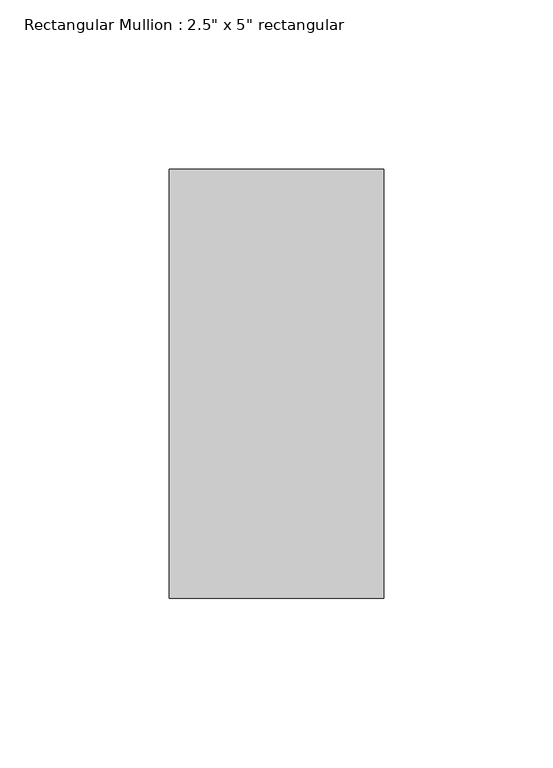
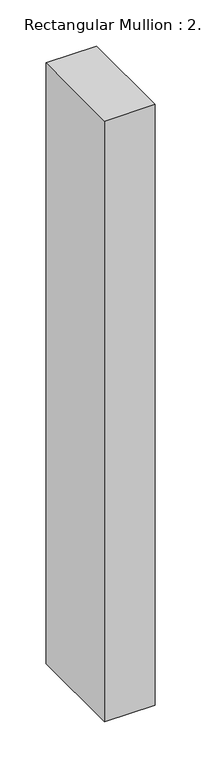
"""IFC4 building model written with IfcOpenShell, lengths in millimetres: member geometry."""

from ifc_helpers import new_model, si_unit, frame, origin, place, context, project, spatial, polyline, outline, extrude, source, transform, mapped, element, save


def member_f14326a3(model_context):
    return source(origin(), model_context, "Body", "SweptSolid", [
        extrude(outline(polyline([(0.0, 63.5), (0.0, -63.5), (-63.5, -63.5), (-63.5, 63.5), (0.0, 63.5)])), frame((0.0, 0.0, -795.8666667), z_axis=(0.0, 0.0, 1.0), x_axis=(1.0, 0.0, 0.0)), (0.0, 0.0, 1.0), 795.8666667),
    ])


if __name__ == "__main__":
    model = new_model("IFC4")
    model_context = context("Model", 3, world=origin())
    ifc_project = project(units=[si_unit("LENGTHUNIT", "METRE", prefix="MILLI")], contexts=[model_context])
    site = spatial("IfcSite", under=ifc_project)
    building = spatial("IfcBuilding", under=site)
    placement = place(None, origin())
    member_shape = member_f14326a3(model_context)
    element("IfcMember", 1, ObjectType="Rectangular Mullion : 2.5\" x 5\" rectangular", at=placement, inside=building, context=model_context, shape_type="MappedRepresentation", body=[
        mapped(member_shape, transform((0.0, 0.0, 0.0), x_axis=(1.0, 0.0, 0.0), y_axis=(0.0, 1.0, 0.0), z_axis=(0.0, 0.0, 1.0))),
    ])
    save(model, "model.ifc")

# Revit data of these elements
# Type "Rectangular Mullion : 2.5\" x 5\" rectangular"
#   built-in parameter 1007304 = 0.416667 (stored number, unit not read)
#   built-in parameter 1007301 = 0.104167 (stored number, unit not read)
#   built-in parameter 1007300 = 0.104167 (stored number, unit not read)
# Element 1 (IfcMember, "Rectangular Mullion : 2.5\" x 5\" rectangular")
#   Materials on its faces: "Aluminum"
# Materials
#   "Aluminum": class "Metal", colour RGB 247 247 247, transparency 0, Description = "Aluminum 6061", Cost = 0
